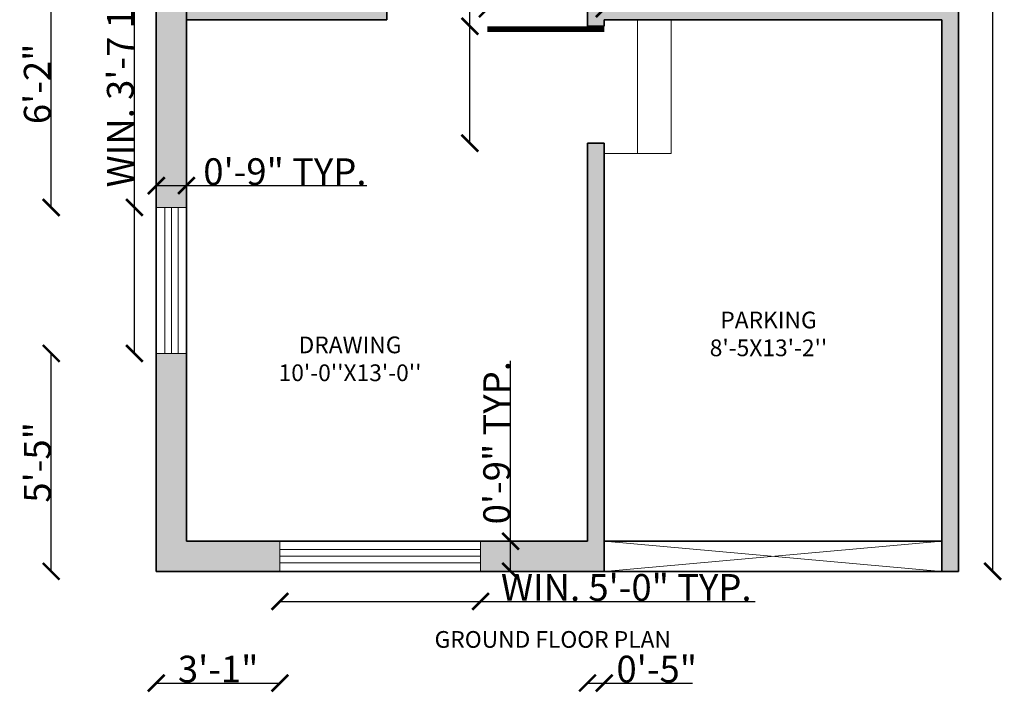
# Model space of a CAD drawing. Units: inches. Extents: x 2267 to 2908, y 1531 to 2136.
# Tile 1 of 5: x 2267 to 2562, y 1551 to 1752. Entities that reach past the tile are written whole.
import ezdxf

# ---------------------------------------------------------------- set-up
doc = ezdxf.new("R2010")
doc.units = ezdxf.units.IN
for name, color, linetype, lineweight in [('A-ANNO-DIMS', 2, 'Continuous', 18), ('A-ANNO-TEXT', 7, 'Continuous', 18), ('A-AREA-IDEN', 7, 'Continuous', 18), ('A-WALL-PATT', 8, 'Continuous', 13), ('DOOR', 30, 'Continuous', 18), ('PARKING', 10, 'Continuous', 18), ('STEPS', 50, 'Continuous', 18), ('WALL', 7, 'Continuous', 35), ('WINDOW', 152, 'Continuous', 18)]:
    doc.layers.add(name, color=color, linetype=linetype, lineweight=lineweight)
doc.styles.get("Standard").update_dxf_attribs({"font": 'arial.ttf'})
doc.dimstyles.get("Standard").update_dxf_attribs({"dimtxt": 8, "dimasz": 5, "dimexe": 0.18, "dimexo": 0.0625, "dimgap": 0.09, "dimtad": 1, "dimdec": 1, "dimzin": 0, "dimdsep": 46, "dimlunit": 4, "dimtxsty": 'Standard', "dimblk": 'ARCHTICK', "dimcen": 0.09, "dimse1": 1, "dimse2": 1, "dimadec": 0, "dimazin": 0, "dimtfac": 1, "dimtdec": 1, "dimtofl": 0, "dimtmove": 0, "dimatfit": 3, "dimfxl": 1, "dimtolj": 1, "dimtzin": 0, "dimarcsym": 0})

# ---------------------------------------------------------------- blocks, each defined once
blk = doc.blocks.new('A$C73484D89')
at = {"layer": 'DOOR'}
blk.add_lwpolyline([(1, 0, 0, 0, 0), (1, 0, 0, 0, 0), (0.975, 0, 0.05, 0.05, 0), (0.975, -1, 0, 0, 0), (0.95, -1, 0, 0, -0.429311), (0, 0, 0, 0, 0), (0, 0, 0, 0, 0)], format="xyseb", dxfattribs=at)
blk = doc.blocks.new('_ArchTick')
at = {"color": 0, "linetype": 'ByBlock', "const_width": 0.15}
blk.add_lwpolyline([(-0.5, -0.5), (0.5, 0.5)], dxfattribs=at)
blk = doc.blocks.new('*D10')
at = {"layer": 'A-ANNO-DIMS', "color": 0, "lineweight": -2, "transparency": 16777216}
blk.add_line((2558.03, 2067.14), (2558.03, 1587.14), dxfattribs=at)
at = {"layer": 'Defpoints', "color": 0, "transparency": 16777216}
for p in [(2547.81, 2067.14), (2547.81, 1587.14), (2558.03, 1587.14)]:
    blk.add_point(p, dxfattribs=at)
at = {"layer": 'A-ANNO-DIMS', "color": 0, "lineweight": -2, "transparency": 16777216, "xscale": 5, "yscale": 5, "zscale": 5}
for p, rotation in [((2558.03, 2067.14), 90), ((2558.03, 1587.14), 270)]:
    blk.add_blockref('_ArchTick', p, dxfattribs=dict(at, rotation=rotation))
at = {"layer": 'A-ANNO-DIMS', "color": 0, "transparency": 16777216, "insert": (2553.86, 1827.14), "char_height": 8, "attachment_point": 5, "rotation": 90}
blk.add_mtext("\\A1;40'", dxfattribs=at)
blk = doc.blocks.new('WIN-60IN')
for p, q in [((0, 6.5), (60, 6.5)), ((0, 4.5), (60, 4.5)), ((0, 2.5), (60, 2.5))]:
    blk.add_line(p, q)
blk.add_lwpolyline([(0, 9), (60, 9), (60, 0), (0, 0)], close=True)
blk = doc.blocks.new('WIN-43_65IN')
for p, q in [((2.5, 0), (2.5, 43.65)), ((4.5, 0), (4.5, 43.65)), ((6.5, 0), (6.5, 43.65))]:
    blk.add_line(p, q)
blk.add_lwpolyline([(0, 0), (0, 43.65), (9, 43.65), (9, 0)], close=True)
blk = doc.blocks.new('*D25')
at = {"layer": 'A-ANNO-DIMS', "color": 0, "lineweight": -2, "transparency": 16777216}
for p, q in [((2401.63, 1750.17), (2401.63, 1819.07)), ((2401.63, 1715.22), (2401.63, 1750.17))]:
    blk.add_line(p, q, dxfattribs=at)
at = {"layer": 'Defpoints', "color": 0, "transparency": 16777216}
for p in [(2401.63, 1750.17), (2406.87, 1750.17), (2406.87, 1715.22)]:
    blk.add_point(p, dxfattribs=at)
at = {"layer": 'A-ANNO-DIMS', "color": 0, "lineweight": -2, "transparency": 16777216, "xscale": 5, "yscale": 5, "zscale": 5}
for p, rotation in [((2401.63, 1750.17), 90), ((2401.63, 1715.22), 270)]:
    blk.add_blockref('_ArchTick', p, dxfattribs=dict(at, rotation=rotation))
at = {"layer": 'A-ANNO-DIMS', "color": 0, "transparency": 16777216, "insert": (2397.4, 1787.12), "char_height": 8, "attachment_point": 5, "rotation": 90}
blk.add_mtext('\\A1;DOOR 2\'-11"', dxfattribs=at)
blk = doc.blocks.new('*D26')
at = {"layer": 'A-ANNO-DIMS', "color": 0, "lineweight": -2, "transparency": 16777216}
blk.add_line((2406.87, 1755.42), (2441.81, 1755.42), dxfattribs=at)
at = {"layer": 'Defpoints', "color": 0, "transparency": 16777216}
for p in [(2441.81, 1755.42), (2406.87, 1750.17), (2441.81, 1750.17)]:
    blk.add_point(p, dxfattribs=at)
at = {"layer": 'A-ANNO-DIMS', "color": 0, "lineweight": -2, "transparency": 16777216, "xscale": 5, "yscale": 5, "zscale": 5, "rotation": 180}
blk.add_blockref('_ArchTick', (2406.87, 1755.42), dxfattribs=at)
at = {"layer": 'A-ANNO-DIMS', "color": 0, "lineweight": -2, "transparency": 16777216, "xscale": 5, "yscale": 5, "zscale": 5}
blk.add_blockref('_ArchTick', (2441.81, 1755.42), dxfattribs=at)
at = {"layer": 'A-ANNO-DIMS', "color": 0, "transparency": 16777216, "insert": (2424.34, 1759.52), "char_height": 8, "attachment_point": 5}
blk.add_mtext('\\A1;2\'-11"', dxfattribs=at)
blk = doc.blocks.new('*D41')
at = {"layer": 'A-ANNO-DIMS', "color": 0, "lineweight": -2, "transparency": 16777216}
for p, q in [((2344.81, 1578.14), (2404.81, 1578.14)), ((2404.81, 1578.14), (2487.01, 1578.14))]:
    blk.add_line(p, q, dxfattribs=at)
at = {"layer": 'Defpoints', "color": 0, "transparency": 16777216}
for p in [(2344.81, 1587.14), (2404.81, 1587.14), (2404.81, 1578.14)]:
    blk.add_point(p, dxfattribs=at)
at = {"layer": 'A-ANNO-DIMS', "color": 0, "lineweight": -2, "transparency": 16777216, "xscale": 5, "yscale": 5, "zscale": 5, "rotation": 180}
blk.add_blockref('_ArchTick', (2344.81, 1578.14), dxfattribs=at)
at = {"layer": 'A-ANNO-DIMS', "color": 0, "lineweight": -2, "transparency": 16777216, "xscale": 5, "yscale": 5, "zscale": 5}
blk.add_blockref('_ArchTick', (2404.81, 1578.14), dxfattribs=at)
at = {"layer": 'A-ANNO-DIMS', "color": 0, "transparency": 16777216, "insert": (2448.41, 1582.32), "char_height": 8, "attachment_point": 5}
blk.add_mtext('\\A1;WIN. 5\'-0" TYP.', dxfattribs=at)
blk = doc.blocks.new('*D42')
at = {"layer": 'A-ANNO-DIMS', "color": 0, "lineweight": -2, "transparency": 16777216}
for p, q in [((2413.81, 1596.14), (2413.81, 1650.09)), ((2413.81, 1587.14), (2413.81, 1596.14))]:
    blk.add_line(p, q, dxfattribs=at)
at = {"layer": 'Defpoints', "color": 0, "transparency": 16777216}
for p in [(2404.81, 1596.14), (2413.81, 1596.14), (2404.81, 1587.14)]:
    blk.add_point(p, dxfattribs=at)
at = {"layer": 'A-ANNO-DIMS', "color": 0, "lineweight": -2, "transparency": 16777216, "xscale": 5, "yscale": 5, "zscale": 5}
for p, rotation in [((2413.81, 1596.14), 90), ((2413.81, 1587.14), 270)]:
    blk.add_blockref('_ArchTick', p, dxfattribs=dict(at, rotation=rotation))
at = {"layer": 'A-ANNO-DIMS', "color": 0, "transparency": 16777216, "insert": (2409.63, 1625.61), "char_height": 8, "attachment_point": 5, "rotation": 90}
blk.add_mtext('\\A1;0\'-9" TYP.', dxfattribs=at)
blk = doc.blocks.new('*D43')
at = {"layer": 'A-ANNO-DIMS', "color": 0, "lineweight": -2, "transparency": 16777216}
for p, q in [((2301.26, 1695.97), (2301.26, 1796.81)), ((2301.26, 1652.32), (2301.26, 1695.97))]:
    blk.add_line(p, q, dxfattribs=at)
at = {"layer": 'Defpoints', "color": 0, "transparency": 16777216}
for p in [(2301.26, 1695.97), (2307.81, 1695.97), (2307.81, 1652.32)]:
    blk.add_point(p, dxfattribs=at)
at = {"layer": 'A-ANNO-DIMS', "color": 0, "lineweight": -2, "transparency": 16777216, "xscale": 5, "yscale": 5, "zscale": 5}
for p, rotation in [((2301.26, 1695.97), 90), ((2301.26, 1652.32), 270)]:
    blk.add_blockref('_ArchTick', p, dxfattribs=dict(at, rotation=rotation))
at = {"layer": 'A-ANNO-DIMS', "color": 0, "transparency": 16777216, "insert": (2297.03, 1748.89), "char_height": 8, "attachment_point": 5, "rotation": 90}
blk.add_mtext('\\A1;WIN. 3\'-7 1/2" TYP.', dxfattribs=at)
blk = doc.blocks.new('*D44')
at = {"layer": 'A-ANNO-DIMS', "color": 0, "lineweight": -2, "transparency": 16777216}
for p, q in [((2307.81, 1702.51), (2316.81, 1702.51)), ((2316.81, 1702.51), (2370.75, 1702.51))]:
    blk.add_line(p, q, dxfattribs=at)
at = {"layer": 'Defpoints', "color": 0, "transparency": 16777216}
for p in [(2316.81, 1702.51), (2307.81, 1695.97), (2316.81, 1695.97)]:
    blk.add_point(p, dxfattribs=at)
at = {"layer": 'A-ANNO-DIMS', "color": 0, "lineweight": -2, "transparency": 16777216, "xscale": 5, "yscale": 5, "zscale": 5, "rotation": 180}
blk.add_blockref('_ArchTick', (2307.81, 1702.51), dxfattribs=at)
at = {"layer": 'A-ANNO-DIMS', "color": 0, "lineweight": -2, "transparency": 16777216, "xscale": 5, "yscale": 5, "zscale": 5}
blk.add_blockref('_ArchTick', (2316.81, 1702.51), dxfattribs=at)
at = {"layer": 'A-ANNO-DIMS', "color": 0, "transparency": 16777216, "insert": (2346.28, 1706.69), "char_height": 8, "attachment_point": 5}
blk.add_mtext('\\A1;0\'-9" TYP.', dxfattribs=at)
blk = doc.blocks.new('*D53')
at = {"layer": 'A-ANNO-DIMS', "color": 0, "lineweight": -2, "transparency": 16777216}
blk.add_line((2307.81, 1553.72), (2344.81, 1553.72), dxfattribs=at)
at = {"layer": 'Defpoints', "color": 0, "transparency": 16777216}
for p in [(2307.81, 1587.14), (2344.81, 1587.14), (2344.81, 1553.72)]:
    blk.add_point(p, dxfattribs=at)
at = {"layer": 'A-ANNO-DIMS', "color": 0, "lineweight": -2, "transparency": 16777216, "xscale": 5, "yscale": 5, "zscale": 5, "rotation": 180}
blk.add_blockref('_ArchTick', (2307.81, 1553.72), dxfattribs=at)
at = {"layer": 'A-ANNO-DIMS', "color": 0, "lineweight": -2, "transparency": 16777216, "xscale": 5, "yscale": 5, "zscale": 5}
blk.add_blockref('_ArchTick', (2344.81, 1553.72), dxfattribs=at)
at = {"layer": 'A-ANNO-DIMS', "color": 0, "transparency": 16777216, "insert": (2326.31, 1557.9), "char_height": 8, "attachment_point": 5}
blk.add_mtext('\\A1;3\'-1"', dxfattribs=at)
blk = doc.blocks.new('*D54')
at = {"layer": 'A-ANNO-DIMS', "color": 0, "lineweight": -2, "transparency": 16777216}
blk.add_line((2276.36, 1587.14), (2276.36, 1652.32), dxfattribs=at)
at = {"layer": 'Defpoints', "color": 0, "transparency": 16777216}
for p in [(2276.36, 1652.32), (2307.81, 1652.32), (2307.81, 1587.14)]:
    blk.add_point(p, dxfattribs=at)
at = {"layer": 'A-ANNO-DIMS', "color": 0, "lineweight": -2, "transparency": 16777216, "xscale": 5, "yscale": 5, "zscale": 5}
for p, rotation in [((2276.36, 1652.32), 90), ((2276.36, 1587.14), 270)]:
    blk.add_blockref('_ArchTick', p, dxfattribs=dict(at, rotation=rotation))
at = {"layer": 'A-ANNO-DIMS', "color": 0, "transparency": 16777216, "insert": (2272.2, 1619.73), "char_height": 8, "attachment_point": 5, "rotation": 90}
blk.add_mtext('\\A1;5\'-5"', dxfattribs=at)
blk = doc.blocks.new('*D55')
at = {"layer": 'A-ANNO-DIMS', "color": 0, "lineweight": -2, "transparency": 16777216}
blk.add_line((2276.36, 1695.97), (2276.36, 1769.93), dxfattribs=at)
at = {"layer": 'Defpoints', "color": 0, "transparency": 16777216}
for p in [(2276.36, 1769.93), (2307.81, 1769.93), (2307.81, 1695.97)]:
    blk.add_point(p, dxfattribs=at)
at = {"layer": 'A-ANNO-DIMS', "color": 0, "lineweight": -2, "transparency": 16777216, "xscale": 5, "yscale": 5, "zscale": 5}
for p, rotation in [((2276.36, 1769.93), 90), ((2276.36, 1695.97), 270)]:
    blk.add_blockref('_ArchTick', p, dxfattribs=dict(at, rotation=rotation))
at = {"layer": 'A-ANNO-DIMS', "color": 0, "transparency": 16777216, "insert": (2272.18, 1732.95), "char_height": 8, "attachment_point": 5, "rotation": 90}
blk.add_mtext('\\A1;6\'-2"', dxfattribs=at)
blk = doc.blocks.new('*D61')
at = {"layer": 'A-ANNO-DIMS', "color": 0, "lineweight": -2, "transparency": 16777216}
for p, q in [((2436.81, 1553.72), (2441.81, 1553.72)), ((2441.81, 1553.72), (2468.25, 1553.72))]:
    blk.add_line(p, q, dxfattribs=at)
at = {"layer": 'Defpoints', "color": 0, "transparency": 16777216}
for p in [(2436.81, 1596.14), (2441.81, 1596.14), (2441.81, 1553.72)]:
    blk.add_point(p, dxfattribs=at)
at = {"layer": 'A-ANNO-DIMS', "color": 0, "lineweight": -2, "transparency": 16777216, "xscale": 5, "yscale": 5, "zscale": 5, "rotation": 180}
blk.add_blockref('_ArchTick', (2436.81, 1553.72), dxfattribs=at)
at = {"layer": 'A-ANNO-DIMS', "color": 0, "lineweight": -2, "transparency": 16777216, "xscale": 5, "yscale": 5, "zscale": 5}
blk.add_blockref('_ArchTick', (2441.81, 1553.72), dxfattribs=at)
at = {"layer": 'A-ANNO-DIMS', "color": 0, "transparency": 16777216, "insert": (2457.53, 1557.9), "char_height": 8, "attachment_point": 5}
blk.add_mtext('\\A1;0\'-5"', dxfattribs=at)

msp = doc.modelspace()

# ---------------------------------------------------------------- hatches: boundary and pattern name
at = {"layer": 'A-WALL-PATT', "transparency": 33554585}
h = msp.add_hatch(color=256, dxfattribs=at)
h.dxf.hatch_style = 1
h.paths.add_polyline_path([(2547.81, 2067.14), (2395.31, 2067.14), (2395.31, 2058.14), (2413.81, 2058.14), (2538.81, 2058.14), (2538.81, 2022.14), (2547.81, 2022.14)])
h.paths.add_polyline_path([(2335.31, 2067.14), (2307.81, 2067.14), (2307.81, 1992.99), (2316.81, 1992.99), (2316.81, 2058.14), (2335.31, 2058.14)])
h.paths.add_polyline_path([(2316.81, 1949.34), (2307.81, 1949.34), (2307.81, 1886.58), (2316.81, 1886.58)])
h.paths.add_polyline_path([(2316.81, 1842.93), (2307.81, 1842.93), (2307.81, 1791.76), (2316.81, 1791.76)])
h.paths.add_polyline_path([(2316.81, 1769.93), (2307.81, 1769.93), (2307.81, 1695.97), (2316.81, 1695.97)])
h.paths.add_polyline_path([(2316.81, 1652.32), (2307.81, 1652.32), (2307.81, 1587.14), (2344.81, 1587.14), (2344.81, 1596.14), (2316.81, 1596.14)])
h.paths.add_polyline_path([(2441.81, 1715.23, -0.025641), (2438.4, 1715.23), (2436.81, 1715.23), (2436.81, 1596.14), (2404.81, 1596.14), (2404.81, 1587.14), (2441.81, 1587.14)])
h.paths.add_polyline_path([(2547.81, 1770.23), (2538.81, 1770.23), (2538.81, 1752.14), (2542.81, 1752.14), (2542.81, 1587.14), (2547.81, 1587.14)])
h.paths.add_polyline_path([(2547.81, 1843.82), (2538.81, 1843.82), (2538.81, 1792.05), (2547.81, 1792.05)])
h.paths.add_polyline_path([(2547.81, 1962.14), (2538.81, 1962.14), (2538.81, 1887.47), (2547.81, 1887.47)])
h.paths.add_polyline_path([(2638.23, 1962.08), (2629.23, 1962.08), (2629.23, 1885.88), (2638.23, 1885.88)])
h.paths.add_polyline_path([(2638.23, 2056.17), (2860.23, 2056.17), (2860.23, 2020.17), (2869.23, 2020.17), (2869.23, 2065.17), (2629.23, 2065.17), (2629.23, 2022.08), (2638.23, 2022.08)])
h.paths.add_polyline_path([(2869.23, 1960.17), (2860.23, 1960.17), (2860.23, 1885.5), (2869.23, 1885.5)])
h.paths.add_polyline_path([(2869.23, 1841.85), (2860.23, 1841.85), (2860.23, 1790.08), (2869.23, 1790.08)])
h.paths.add_polyline_path([(2869.23, 1768.26), (2860.23, 1768.26), (2860.23, 1768.05), (2860.23, 1720.44), (2869.23, 1720.44)])
h.paths.add_polyline_path([(2869.23, 1660.44), (2860.23, 1660.44), (2860.23, 1585.17), (2869.23, 1585.17)])
h.paths.add_polyline_path([(2763.23, 1594.17), (2726.23, 1594.17), (2726.23, 1585.17), (2763.23, 1585.17)])
h.paths.add_polyline_path([(2666.23, 1594.17), (2638.23, 1594.17), (2638.23, 1768.3), (2629.23, 1768.3), (2629.23, 1585.17), (2666.23, 1585.17)])
h.paths.add_polyline_path([(2638.23, 1842.24), (2629.23, 1842.24), (2629.23, 1790.12), (2638.23, 1790.12)])
h = msp.add_hatch(color=256, dxfattribs=at)
h.dxf.hatch_style = 1
h.paths.add_polyline_path([(2763.23, 1755.17), (2758.23, 1755.17), (2758.23, 1625.17), (2760.21, 1625.17, -0.025641), (2763.23, 1625.17)])
h.paths.add_polyline_path([(2638.23, 1750.17), (2679.86, 1750.17, -0.025641), (2679.86, 1752.99), (2679.86, 1755.17), (2638.23, 1755.17)])
h.paths.add_polyline_path([(2860.23, 1625.17), (2860.23, 1630.17), (2796.25, 1630.17), (2796.25, 1628.39, -0.025641), (2796.25, 1625.17)])
h.paths.add_polyline_path([(2730.26, 1919.17), (2745.45, 1919.17), (2745.45, 1924.17), (2740.23, 1924.17), (2740.23, 2056.17), (2735.23, 2056.17), (2735.23, 1924.17), (2730.26, 1924.17)])
h.paths.add_polyline_path([(2860.23, 1919.17), (2860.23, 1924.17), (2774.38, 1924.17), (2774.38, 1921.99, -0.025641), (2774.38, 1919.17)])
h.paths.add_polyline_path([(2638.23, 1919.17), (2701.33, 1919.17, -0.025641), (2701.33, 1921.99), (2701.33, 1924.17), (2638.23, 1924.17)])
h.paths.add_polyline_path([(2538.81, 1752.14), (2538.81, 1757.14), (2441.81, 1757.14), (2441.81, 1762.09), (2439.73, 1762.09, -0.025641), (2436.81, 1762.09), (2436.81, 1750.17), (2441.81, 1750.17), (2441.81, 1752.14)])
h.paths.add_polyline_path([(2436.81, 1810.14), (2436.81, 1792.08), (2441.81, 1792.08), (2441.81, 1805.14), (2538.81, 1805.14), (2538.81, 1810.14)])
h.paths.add_polyline_path([(2346.81, 1805.14), (2346.81, 1810.14), (2316.81, 1810.14), (2316.81, 1805.14)], flags=0)
h.paths.add_polyline_path([(2376.81, 1810.14), (2371.81, 1810.14), (2371.81, 1757.14), (2316.81, 1757.14), (2316.81, 1752.14), (2376.81, 1752.14)])
h.paths.add_polyline_path([(2374.47, 1921.14), (2374.47, 1926.14), (2316.81, 1926.14), (2316.81, 1921.14)])
h.paths.add_polyline_path([(2413.81, 1921.14), (2421.94, 1921.14), (2421.94, 1926.14), (2418.81, 1926.14), (2418.81, 2058.14), (2413.81, 2058.14)])
h.paths.add_polyline_path([(2316.81, 2022.14), (2316.81, 2017.14), (2381.27, 2017.14), (2381.27, 2022.14)])
h.paths.add_polyline_path([(2455.63, 1926.14), (2455.63, 1924.43, -0.025641), (2455.63, 1921.14), (2538.81, 1921.14), (2538.81, 1926.14)])

# ---------------------------------------------------------------- linework, layer by layer
at = {"layer": 'PARKING'}
for p, q in [((2441.81, 1587.14), (2542.81, 1596.14)), ((2441.81, 1596.14), (2542.81, 1587.14))]:
    msp.add_line(p, q, dxfattribs=at)
at = {"layer": 'STEPS'}
for p, q in [((2451.81, 1712.14), (2451.81, 1752.14)), ((2461.81, 1752.14), (2461.81, 1712.14)), ((2461.81, 1712.14), (2441.81, 1712.14))]:
    msp.add_line(p, q, dxfattribs=at)
at = {"layer": 'WALL'}
for p, q in [((2307.81, 2067.14), (2307.81, 1587.14)), ((2547.81, 2067.14), (2547.81, 1587.14)), ((2316.81, 2058.14), (2316.81, 1596.14)), ((2376.81, 1810.14), (2376.81, 1752.14)), ((2436.81, 1810.14), (2436.81, 1750.17)), ((2316.81, 1752.14), (2376.81, 1752.14)), ((2441.81, 1750.17), (2436.81, 1750.17)), ((2441.81, 1752.14), (2538.81, 1752.14)), ((2441.81, 1752.14), (2441.81, 1750.17)), ((2538.81, 1752.14), (2542.81, 1752.14)), ((2542.81, 1752.14), (2542.81, 1587.14)), ((2436.81, 1715.23), (2436.81, 1596.14)), ((2436.81, 1715.23), (2441.81, 1715.23)), ((2441.81, 1715.23), (2441.81, 1587.14)), ((2316.81, 1596.14), (2436.81, 1596.14)), ((2441.81, 1596.14), (2542.81, 1596.14)), ((2307.81, 1587.14), (2547.81, 1587.14))]:
    msp.add_line(p, q, dxfattribs=at)

# ---------------------------------------------------------------- block references
at = {"layer": 'DOOR', "xscale": -34.9390340430292, "yscale": 34.9390340430292, "zscale": 34.9390340430292, "rotation": 270}
msp.add_blockref('A$C73484D89', (2441.81, 1715.23), dxfattribs=at)
at = {"layer": 'WINDOW'}
for name, p in [('WIN-43_65IN', (2307.81, 1652.32)), ('WIN-60IN', (2344.81, 1587.14))]:
    msp.add_blockref(name, p, dxfattribs=at)

# ---------------------------------------------------------------- texts
at = {"layer": 'A-ANNO-TEXT', "insert": (2379.65, 1569.27), "char_height": 5, "attachment_point": 1}
msp.add_mtext_dynamic_manual_height_columns('\\pxqc;GROUND FLOOR PLAN', width=93.5369, gutter_width=12.5, heights=[0], dxfattribs=at)
at = {"layer": 'A-AREA-IDEN', "char_height": 5, "attachment_point": 1}
for s, insert in [("\\pxqc;PARKING\\P8'-5X13'-2''", (2470.26, 1664.82)), ("\\pxqc;DRAWING\\P10'-0''X13'-0''", (2345.06, 1657.37))]:
    msp.add_mtext_dynamic_manual_height_columns(s, width=41.4104, gutter_width=12.5, heights=[0], dxfattribs=dict(at, insert=insert))

# ---------------------------------------------------------------- dimensions: what is measured, and where the dimension line sits
at = {"layer": 'A-ANNO-DIMS'}
for base, p1, p2, override, picture, middle in [((2558.03, 1587.14), (2547.81, 2067.14), (2547.81, 1587.14), {"dimclrd": 0, "dimclre": 0, "dimclrt": 0}, '*D10', (2553.86, 1827.14)), ((2276.36, 1769.93), (2307.81, 1695.97), (2307.81, 1769.93), {"dimdec": 1, "dimlfac": 1, "dimrnd": 0, "dimzin": 1, "dimdsep": 46, "dimlunit": 4, "dimfrac": 2}, '*D55', (2272.18, 1732.95)), ((2276.36, 1652.32), (2307.81, 1587.14), (2307.81, 1652.32), {"dimdec": 1, "dimlfac": 1, "dimrnd": 0, "dimzin": 1, "dimdsep": 46, "dimlunit": 4, "dimfrac": 2}, '*D54', (2272.2, 1619.73))]:
    dim = msp.add_linear_dim(base=base, p1=p1, p2=p2, angle=90, dimstyle='Standard', override=override, dxfattribs=at)
    dim.commit()
    dim.dimension.update_dxf_attribs({"geometry": picture, "text_midpoint": middle})
for base, p1, p2, text, picture, middle in [((2401.6262, 1750.1728), (2406.8687, 1715.2225), (2406.8687, 1750.1728), 'DOOR <>', '*D25', (2397.397, 1787.1209)), ((2301.2607, 1695.9659), (2307.8078, 1652.319), (2307.8078, 1695.9659), 'WIN. <> TYP.', '*D43', (2297.0316, 1748.8895)), ((2413.81, 1596.14), (2404.81, 1587.14), (2404.81, 1596.14), '<> TYP.', '*D42', (2409.63, 1625.61))]:
    dim = msp.add_linear_dim(base=base, p1=p1, p2=p2, angle=90, text=text, dimstyle='Standard', override={"dimdec": 1, "dimlfac": 1, "dimrnd": 0, "dimzin": 1, "dimdsep": 46, "dimlunit": 4, "dimfrac": 2}, dxfattribs=at)
    dim.commit()
    dim.dimension.update_dxf_attribs({"geometry": picture, "text_midpoint": middle})
for base, p1, p2, picture, middle in [((2441.81, 1755.42), (2406.87, 1750.17), (2441.81, 1750.17), '*D26', (2424.34, 1759.52)), ((2441.81, 1553.72), (2436.81, 1596.14), (2441.81, 1596.14), '*D61', (2457.53, 1557.9)), ((2344.81, 1553.72), (2307.81, 1587.14), (2344.81, 1587.14), '*D53', (2326.31, 1557.9))]:
    dim = msp.add_linear_dim(base=base, p1=p1, p2=p2, dimstyle='Standard', override={"dimdec": 1, "dimlfac": 1, "dimrnd": 0, "dimzin": 1, "dimdsep": 46, "dimlunit": 4, "dimfrac": 2}, dxfattribs=at)
    dim.commit()
    dim.dimension.update_dxf_attribs({"geometry": picture, "text_midpoint": middle})
for base, p1, p2, text, picture, middle in [((2316.81, 1702.51), (2307.81, 1695.97), (2316.81, 1695.97), '<> TYP.', '*D44', (2346.28, 1706.69)), ((2404.81, 1578.14), (2344.81, 1587.14), (2404.81, 1587.14), 'WIN. <> TYP.', '*D41', (2448.41, 1582.32))]:
    dim = msp.add_linear_dim(base=base, p1=p1, p2=p2, text=text, dimstyle='Standard', override={"dimdec": 1, "dimlfac": 1, "dimrnd": 0, "dimzin": 1, "dimdsep": 46, "dimlunit": 4, "dimfrac": 2}, dxfattribs=at)
    dim.commit()
    dim.dimension.update_dxf_attribs({"geometry": picture, "text_midpoint": middle})

doc.saveas('drawing.dxf')
